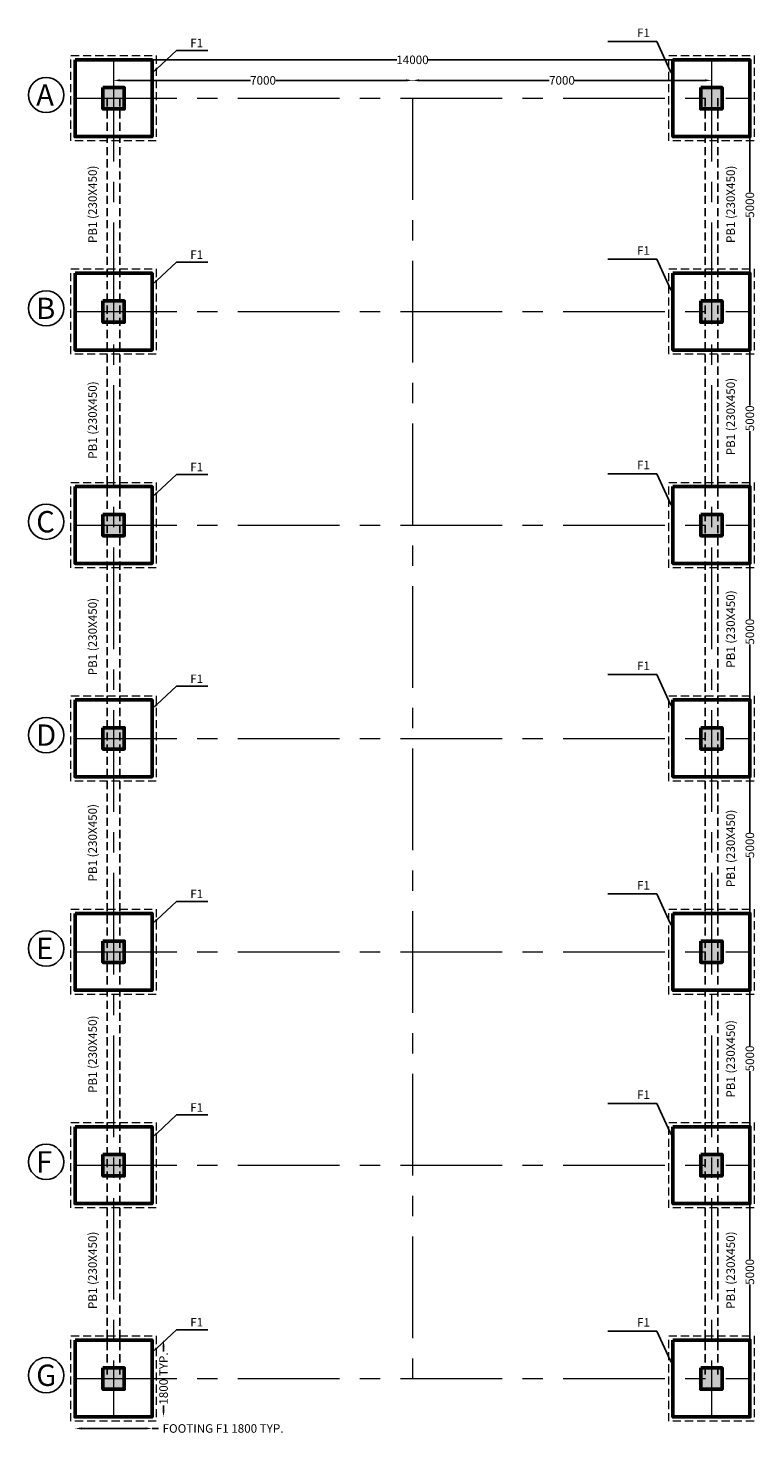
# Model space of a CAD drawing. Units: millimetres. Extents: x -106221 to -52078, y 251365 to 289027.
# Tile 1 of 2: x -106221 to -89199, y 251365 to 284801. Entities that reach past the tile are written whole.
import ezdxf
from ezdxf import colors
from ezdxf.entities.mleader import LeaderData, LeaderLine
from ezdxf.math import Vec2, Vec3

# ---------------------------------------------------------------- set-up
doc = ezdxf.new("R2010")
doc.units = ezdxf.units.MM
doc.header["$LTSCALE"] = 15
doc.header["$MEASUREMENT"] = 0
doc.linetypes.add('CENTER', pattern=[50.8, 31.75, -6.35, 6.35, -6.35])
doc.linetypes.add('DASHED', pattern=[19.05, 12.7, -6.35])
for name, color, linetype, lineweight in [('S-ANNO-DIMS', 2, 'Continuous', 18), ('S-ANNO-TEXT', 7, 'Continuous', 25), ('S-BEAM', 3, 'DASHED', 25), ('S-FNDN', 7, 'Continuous', 50), ('S-FNDN-PCC', 8, 'DASHED', 18), ('S-GRID', 8, 'CENTER', 18), ('S-GRID-IDEN', 7, 'Continuous', 25)]:
    doc.layers.add(name, color=color, linetype=linetype, lineweight=lineweight)
doc.styles.get("Standard").update_dxf_attribs({"font": 'arial.ttf'})
doc.dimstyles.get("Standard").update_dxf_attribs({"dimtxt": 200, "dimasz": 150, "dimexe": 0.18, "dimexo": 0.0625, "dimgap": 0.09, "dimtad": 0, "dimdec": 0, "dimzin": 0, "dimdsep": 46, "dimtxsty": 'Standard', "dimcen": 0.09, "dimadec": 0, "dimazin": 0, "dimtfac": 1, "dimtdec": 0, "dimtofl": 0, "dimtmove": 0, "dimatfit": 3, "dimfxl": 1, "dimfxlon": 1, "dimtolj": 1, "dimtzin": 0, "dimarcsym": 0})

# ---------------------------------------------------------------- blocks, each defined once
blk = doc.blocks.new('*D1')
at = {"layer": 'Defpoints', "color": 0, "ltscale": 15, "transparency": 16777216}
for p in [(-104230, 284068), (-90230, 284068), (-90230, 284068)]:
    blk.add_point(p, dxfattribs=at)
at = {"layer": 'S-ANNO-DIMS', "color": 0, "lineweight": -2, "ltscale": 15, "transparency": 16777216}
for p, q in [((-104230, 284068), (-104230, 284068)), ((-104080, 284068), (-97596, 284068)), ((-90380, 284068), (-96863, 284068)), ((-90230, 284068), (-90230, 284068))]:
    blk.add_line(p, q, dxfattribs=at)
at = {"layer": 'S-ANNO-DIMS', "color": 0, "ltscale": 15, "transparency": 16777216}
for points in [[(-104080, 284093), (-104080, 284043), (-104230, 284068)], [(-90380, 284093), (-90380, 284043), (-90230, 284068)]]:
    blk.add_solid(points, dxfattribs=at)
at = {"layer": 'S-ANNO-DIMS', "color": 0, "ltscale": 15, "transparency": 16777216, "insert": (-97230, 284068), "char_height": 200, "attachment_point": 5}
blk.add_mtext('\\A1;14000', dxfattribs=at)
blk = doc.blocks.new('*D2')
at = {"layer": 'Defpoints', "color": 0, "ltscale": 15, "transparency": 16777216}
for p in [(-104230, 283539), (-97230, 283587), (-97230, 283168)]:
    blk.add_point(p, dxfattribs=at)
at = {"layer": 'S-ANNO-DIMS', "color": 0, "lineweight": -2, "ltscale": 15, "transparency": 16777216}
for p, q in [((-104230, 283586), (-104230, 283587)), ((-104080, 283587), (-101027, 283587)), ((-97380, 283587), (-100432, 283587)), ((-97230, 283586), (-97230, 283587))]:
    blk.add_line(p, q, dxfattribs=at)
at = {"layer": 'S-ANNO-DIMS', "color": 0, "ltscale": 15, "transparency": 16777216}
for points in [[(-104080, 283612), (-104080, 283562), (-104230, 283587)], [(-97380, 283612), (-97380, 283562), (-97230, 283587)]]:
    blk.add_solid(points, dxfattribs=at)
at = {"layer": 'S-ANNO-DIMS', "color": 0, "ltscale": 15, "transparency": 16777216, "insert": (-100730, 283587), "char_height": 200, "attachment_point": 5}
blk.add_mtext('\\A1;7000', dxfattribs=at)
blk = doc.blocks.new('*D3')
at = {"layer": 'Defpoints', "color": 0, "ltscale": 15, "transparency": 16777216}
for p in [(-90230, 283587), (-90230, 283418), (-97230, 283168)]:
    blk.add_point(p, dxfattribs=at)
at = {"layer": 'S-ANNO-DIMS', "color": 0, "lineweight": -2, "ltscale": 15, "transparency": 16777216}
for p, q in [((-97230, 283586), (-97230, 283588)), ((-97080, 283587), (-94027, 283587)), ((-90380, 283587), (-93432, 283587)), ((-90230, 283586), (-90230, 283588))]:
    blk.add_line(p, q, dxfattribs=at)
at = {"layer": 'S-ANNO-DIMS', "color": 0, "ltscale": 15, "transparency": 16777216}
for points in [[(-97080, 283612), (-97080, 283562), (-97230, 283587)], [(-90380, 283612), (-90380, 283562), (-90230, 283587)]]:
    blk.add_solid(points, dxfattribs=at)
at = {"layer": 'S-ANNO-DIMS', "color": 0, "ltscale": 15, "transparency": 16777216, "insert": (-93730, 283587), "char_height": 200, "attachment_point": 5}
blk.add_mtext('\\A1;7000', dxfattribs=at)
blk = doc.blocks.new('*D4')
at = {"layer": 'Defpoints', "color": 0, "ltscale": 15, "transparency": 16777216}
for p in [(-89330, 283168), (-89330, 278168), (-89330, 278168)]:
    blk.add_point(p, dxfattribs=at)
at = {"layer": 'S-ANNO-DIMS', "color": 0, "lineweight": -2, "ltscale": 15, "transparency": 16777216}
for p, q in [((-89330, 283168), (-89330, 283168)), ((-89330, 283018), (-89330, 280966)), ((-89330, 278318), (-89330, 280369)), ((-89330, 278168), (-89330, 278168))]:
    blk.add_line(p, q, dxfattribs=at)
at = {"layer": 'S-ANNO-DIMS', "color": 0, "ltscale": 15, "transparency": 16777216}
for points in [[(-89355, 283018), (-89305, 283018), (-89330, 283168)], [(-89355, 278318), (-89305, 278318), (-89330, 278168)]]:
    blk.add_solid(points, dxfattribs=at)
at = {"layer": 'S-ANNO-DIMS', "color": 0, "ltscale": 15, "transparency": 16777216, "insert": (-89330, 280668), "char_height": 200, "attachment_point": 5, "rotation": 90}
blk.add_mtext('\\A1;5000', dxfattribs=at)
blk = doc.blocks.new('*D5')
at = {"layer": 'Defpoints', "color": 0, "ltscale": 15, "transparency": 16777216}
for p in [(-89330, 278168), (-89330, 273168), (-89330, 273168)]:
    blk.add_point(p, dxfattribs=at)
at = {"layer": 'S-ANNO-DIMS', "color": 0, "lineweight": -2, "ltscale": 15, "transparency": 16777216}
for p, q in [((-89330, 278168), (-89330, 278168)), ((-89330, 278018), (-89330, 275966)), ((-89330, 273318), (-89330, 275369)), ((-89330, 273168), (-89330, 273168))]:
    blk.add_line(p, q, dxfattribs=at)
at = {"layer": 'S-ANNO-DIMS', "color": 0, "ltscale": 15, "transparency": 16777216}
for points in [[(-89355, 278018), (-89305, 278018), (-89330, 278168)], [(-89355, 273318), (-89305, 273318), (-89330, 273168)]]:
    blk.add_solid(points, dxfattribs=at)
at = {"layer": 'S-ANNO-DIMS', "color": 0, "ltscale": 15, "transparency": 16777216, "insert": (-89330, 275668), "char_height": 200, "attachment_point": 5, "rotation": 90}
blk.add_mtext('\\A1;5000', dxfattribs=at)
blk = doc.blocks.new('*D6')
at = {"layer": 'Defpoints', "color": 0, "ltscale": 15, "transparency": 16777216}
for p in [(-89330, 273168), (-89330, 268168), (-89330, 268168)]:
    blk.add_point(p, dxfattribs=at)
at = {"layer": 'S-ANNO-DIMS', "color": 0, "lineweight": -2, "ltscale": 15, "transparency": 16777216}
for p, q in [((-89330, 273168), (-89330, 273168)), ((-89330, 273018), (-89330, 270966)), ((-89330, 268318), (-89330, 270369)), ((-89330, 268168), (-89330, 268168))]:
    blk.add_line(p, q, dxfattribs=at)
at = {"layer": 'S-ANNO-DIMS', "color": 0, "ltscale": 15, "transparency": 16777216}
for points in [[(-89355, 273018), (-89305, 273018), (-89330, 273168)], [(-89355, 268318), (-89305, 268318), (-89330, 268168)]]:
    blk.add_solid(points, dxfattribs=at)
at = {"layer": 'S-ANNO-DIMS', "color": 0, "ltscale": 15, "transparency": 16777216, "insert": (-89330, 270668), "char_height": 200, "attachment_point": 5, "rotation": 90}
blk.add_mtext('\\A1;5000', dxfattribs=at)
blk = doc.blocks.new('*D7')
at = {"layer": 'Defpoints', "color": 0, "ltscale": 15, "transparency": 16777216}
for p in [(-89330, 268168), (-89330, 263168), (-89330, 263168)]:
    blk.add_point(p, dxfattribs=at)
at = {"layer": 'S-ANNO-DIMS', "color": 0, "lineweight": -2, "ltscale": 15, "transparency": 16777216}
for p, q in [((-89330, 268168), (-89330, 268168)), ((-89330, 268018), (-89330, 265966)), ((-89330, 263318), (-89330, 265369)), ((-89330, 263168), (-89330, 263168))]:
    blk.add_line(p, q, dxfattribs=at)
at = {"layer": 'S-ANNO-DIMS', "color": 0, "ltscale": 15, "transparency": 16777216}
for points in [[(-89355, 268018), (-89305, 268018), (-89330, 268168)], [(-89355, 263318), (-89305, 263318), (-89330, 263168)]]:
    blk.add_solid(points, dxfattribs=at)
at = {"layer": 'S-ANNO-DIMS', "color": 0, "ltscale": 15, "transparency": 16777216, "insert": (-89330, 265668), "char_height": 200, "attachment_point": 5, "rotation": 90}
blk.add_mtext('\\A1;5000', dxfattribs=at)
blk = doc.blocks.new('*D8')
at = {"layer": 'Defpoints', "color": 0, "ltscale": 15, "transparency": 16777216}
for p in [(-89330, 263168), (-89330, 258168), (-89330, 258168)]:
    blk.add_point(p, dxfattribs=at)
at = {"layer": 'S-ANNO-DIMS', "color": 0, "lineweight": -2, "ltscale": 15, "transparency": 16777216}
for p, q in [((-89330, 263168), (-89330, 263168)), ((-89330, 263018), (-89330, 260966)), ((-89330, 258318), (-89330, 260369)), ((-89330, 258168), (-89330, 258168))]:
    blk.add_line(p, q, dxfattribs=at)
at = {"layer": 'S-ANNO-DIMS', "color": 0, "ltscale": 15, "transparency": 16777216}
for points in [[(-89355, 263018), (-89305, 263018), (-89330, 263168)], [(-89355, 258318), (-89305, 258318), (-89330, 258168)]]:
    blk.add_solid(points, dxfattribs=at)
at = {"layer": 'S-ANNO-DIMS', "color": 0, "ltscale": 15, "transparency": 16777216, "insert": (-89330, 260668), "char_height": 200, "attachment_point": 5, "rotation": 90}
blk.add_mtext('\\A1;5000', dxfattribs=at)
blk = doc.blocks.new('*D9')
at = {"layer": 'Defpoints', "color": 0, "ltscale": 15, "transparency": 16777216}
for p in [(-89330, 258168), (-89330, 253168), (-89330, 253168)]:
    blk.add_point(p, dxfattribs=at)
at = {"layer": 'S-ANNO-DIMS', "color": 0, "lineweight": -2, "ltscale": 15, "transparency": 16777216}
for p, q in [((-89330, 258168), (-89330, 258168)), ((-89330, 258018), (-89330, 255966)), ((-89330, 253318), (-89330, 255369)), ((-89330, 253168), (-89330, 253168))]:
    blk.add_line(p, q, dxfattribs=at)
at = {"layer": 'S-ANNO-DIMS', "color": 0, "ltscale": 15, "transparency": 16777216}
for points in [[(-89355, 258018), (-89305, 258018), (-89330, 258168)], [(-89355, 253318), (-89305, 253318), (-89330, 253168)]]:
    blk.add_solid(points, dxfattribs=at)
at = {"layer": 'S-ANNO-DIMS', "color": 0, "ltscale": 15, "transparency": 16777216, "insert": (-89330, 255668), "char_height": 200, "attachment_point": 5, "rotation": 90}
blk.add_mtext('\\A1;5000', dxfattribs=at)
blk = doc.blocks.new('FOOTING-F1')
h = blk.add_hatch(color=256)
h.dxf.hatch_style = 1
h.paths.add_polyline_path([(1150, 1150), (650, 1150), (650, 650), (1150, 650)])
for points in [[(0, 1800), (1800, 1800), (1800, 0), (0, 0)], [(650, 1150), (1150, 1150), (1150, 650), (650, 650)]]:
    blk.add_lwpolyline(points, close=True)
blk = doc.blocks.new('*D13')
at = {"layer": 'Defpoints', "color": 0, "ltscale": 15, "transparency": 16777216}
for p in [(-105130, 252268), (-103330, 252268), (-103330, 251998)]:
    blk.add_point(p, dxfattribs=at)
at = {"layer": 'S-ANNO-DIMS', "color": 0, "lineweight": -2, "ltscale": 15, "transparency": 16777216}
for p, q in [((-105130, 251999), (-105130, 251997)), ((-104980, 251998), (-103480, 251998)), ((-103330, 251999), (-103330, 251997)), ((-103330, 251998), (-103180, 251998))]:
    blk.add_line(p, q, dxfattribs=at)
at = {"layer": 'S-ANNO-DIMS', "color": 0, "ltscale": 15, "transparency": 16777216}
for points in [[(-104980, 252023), (-104980, 251973), (-105130, 251998)], [(-103480, 252023), (-103480, 251973), (-103330, 251998)]]:
    blk.add_solid(points, dxfattribs=at)
at = {"layer": 'S-ANNO-DIMS', "color": 0, "ltscale": 15, "transparency": 16777216, "insert": (-101666, 251998), "char_height": 200, "attachment_point": 5}
blk.add_mtext('\\A1;FOOTING F1 1800 TYP.', dxfattribs=at)
blk = doc.blocks.new('*D14')
at = {"layer": 'Defpoints', "color": 0, "ltscale": 15, "transparency": 16777216}
for p in [(-103330, 254068), (-103060, 254068), (-103330, 252268)]:
    blk.add_point(p, dxfattribs=at)
at = {"layer": 'S-ANNO-DIMS', "color": 0, "lineweight": -2, "ltscale": 15, "transparency": 16777216}
for p, q in [((-103061, 254068), (-103060, 254068)), ((-103060, 253918), (-103060, 253800)), ((-103060, 252418), (-103060, 252535)), ((-103061, 252268), (-103060, 252268))]:
    blk.add_line(p, q, dxfattribs=at)
at = {"layer": 'S-ANNO-DIMS', "color": 0, "ltscale": 15, "transparency": 16777216}
for points in [[(-103085, 253918), (-103035, 253918), (-103060, 254068)], [(-103085, 252418), (-103035, 252418), (-103060, 252268)]]:
    blk.add_solid(points, dxfattribs=at)
at = {"layer": 'S-ANNO-DIMS', "color": 0, "ltscale": 15, "transparency": 16777216, "insert": (-103060, 253168), "char_height": 200, "attachment_point": 5, "rotation": 90}
blk.add_mtext('\\A1;1800 TYP.', dxfattribs=at)

msp = doc.modelspace()

# ---------------------------------------------------------------- linework, layer by layer
at = {"layer": 'S-BEAM'}
for p, q in [((-104379.8, 283167.6), (-104379.8, 253167.6)), ((-104079.8, 283167.6), (-104079.8, 253167.6)), ((-90379.8, 283167.6), (-90379.8, 253167.6)), ((-90079.8, 283167.6), (-90079.8, 253167.6))]:
    msp.add_line(p, q, dxfattribs=at)
at = {"layer": 'S-FNDN-PCC'}
for points in [[(-105229.8, 284167.6), (-103229.8, 284167.6), (-103229.8, 282167.6), (-105229.8, 282167.6)], [(-91229.8, 284167.6), (-89229.8, 284167.6), (-89229.8, 282167.6), (-91229.8, 282167.6)], [(-105229.8, 279167.6), (-103229.8, 279167.6), (-103229.8, 277167.6), (-105229.8, 277167.6)], [(-91229.8, 279167.6), (-89229.8, 279167.6), (-89229.8, 277167.6), (-91229.8, 277167.6)], [(-105229.8, 274167.6), (-103229.8, 274167.6), (-103229.8, 272167.6), (-105229.8, 272167.6)], [(-91229.8, 274167.6), (-89229.8, 274167.6), (-89229.8, 272167.6), (-91229.8, 272167.6)], [(-105229.8, 269167.6), (-103229.8, 269167.6), (-103229.8, 267167.6), (-105229.8, 267167.6)], [(-91229.8, 269167.6), (-89229.8, 269167.6), (-89229.8, 267167.6), (-91229.8, 267167.6)], [(-105229.8, 264167.6), (-103229.8, 264167.6), (-103229.8, 262167.6), (-105229.8, 262167.6)], [(-91229.8, 264167.6), (-89229.8, 264167.6), (-89229.8, 262167.6), (-91229.8, 262167.6)], [(-105229.8, 259167.6), (-103229.8, 259167.6), (-103229.8, 257167.6), (-105229.8, 257167.6)], [(-91229.8, 259167.6), (-89229.8, 259167.6), (-89229.8, 257167.6), (-91229.8, 257167.6)], [(-105229.8, 254167.6), (-103229.8, 254167.6), (-103229.8, 252167.6), (-105229.8, 252167.6)], [(-91229.8, 254167.6), (-89229.8, 254167.6), (-89229.8, 252167.6), (-91229.8, 252167.6)]]:
    msp.add_lwpolyline(points, close=True, dxfattribs=at)
at = {"layer": 'S-GRID', "ltscale": 5}
for p, q in [((-104229.8, 284067.6), (-104229.8, 252267.6)), ((-90229.8, 284067.6), (-90229.8, 252267.6)), ((-105129.8, 283167.6), (-89329.8, 283167.6)), ((-97229.8, 283167.6), (-97229.8, 253167.6)), ((-105129.8, 278167.6), (-89329.8, 278167.6)), ((-105129.8, 273167.6), (-89329.8, 273167.6)), ((-105129.8, 268167.6), (-89329.8, 268167.6)), ((-105129.8, 263167.6), (-89329.8, 263167.6)), ((-105129.8, 258167.6), (-89329.8, 258167.6)), ((-105129.8, 253167.6), (-89329.8, 253167.6))]:
    msp.add_line(p, q, dxfattribs=at)
at = {"layer": 'S-GRID-IDEN', "ltscale": 15}
for centre in [(-105808.1, 283244.8), (-105808.1, 278244.8), (-105808.1, 273244.8), (-105808.1, 268244.8), (-105808.1, 263244.8), (-105808.1, 258244.8), (-105808.1, 253244.8)]:
    msp.add_circle(centre, 412.7, dxfattribs=at)

# ---------------------------------------------------------------- block references
at = {"layer": 'S-FNDN'}
for p in [(-105129.8, 282267.6), (-91129.8, 282267.6), (-105129.8, 277267.6), (-91129.8, 277267.6), (-105129.8, 272267.6), (-91129.8, 272267.6), (-105129.8, 267267.6), (-91129.8, 267267.6), (-105129.8, 262267.6), (-91129.8, 262267.6), (-105129.8, 257267.6), (-91129.8, 257267.6), (-105129.8, 252267.6), (-91129.8, 252267.6)]:
    msp.add_blockref('FOOTING-F1', p, dxfattribs=at)

# ---------------------------------------------------------------- texts
at = {"layer": 'S-ANNO-TEXT', "ltscale": 15, "char_height": 200, "attachment_point": 1}
for insert in [(-102433.5, 284563.6), (-91971.3, 284801.1), (-102433.5, 279602.9), (-91971.3, 279699.1), (-102433.5, 274625.6), (-91971.3, 274673.2), (-91971.3, 269967.3), (-102433.5, 269664.7), (-91971.3, 264826.8), (-102433.5, 264624.6), (-91971.3, 259917.2), (-102433.5, 259619.1), (-102433.5, 254587.4), (-91971.3, 254582.9)]:
    msp.add_mtext_dynamic_manual_height_columns('F1', width=2119.366, gutter_width=1, heights=[262.2], dxfattribs=dict(at, insert=insert))
at = {"layer": 'S-ANNO-TEXT', "ltscale": 15, "char_height": 200, "attachment_point": 1, "rotation": 90}
for insert in [(-104821.9, 279775.3), (-89879.1, 279775.3), (-89879.1, 274801.3), (-104821.9, 274720.4), (-89879.1, 269822.9), (-104821.9, 269645.2), (-104821.9, 264816), (-89879.1, 264683.7), (-104821.9, 259859.8), (-89879.1, 259750.9), (-104821.9, 254796), (-89879.1, 254800.4)]:
    msp.add_mtext_dynamic_manual_height_columns('PB1 (230X450)', width=2119.366, gutter_width=1, heights=[0], dxfattribs=dict(at, insert=insert))
at = {"layer": 'S-GRID-IDEN', "ltscale": 15, "char_height": 500, "attachment_point": 1}
for s, insert in [('A', (-106041.6, 283494.8)), ('B', (-106041.6, 278494.8)), ('C', (-106041.6, 273494.8)), ('D', (-106041.6, 268494.8)), ('E', (-106041.6, 263494.8)), ('F', (-106041.6, 258494.8)), ('G', (-106041.6, 253494.8))]:
    msp.add_mtext_dynamic_manual_height_columns(s, width=500, gutter_width=1, heights=[0], dxfattribs=dict(at, insert=insert))

# ---------------------------------------------------------------- dimensions: what is measured, and where the dimension line sits
at = {"layer": 'S-ANNO-DIMS', "ltscale": 15}
for base, p1, p2, picture, middle in [((-90229.8, 284067.6), (-104229.8, 284067.6), (-90229.8, 284067.6), '*D1', (-97229.8, 284067.6)), ((-97229.8, 283587.3), (-104229.8, 283538.9), (-97229.8, 283167.6), '*D2', (-100729.8, 283587.3)), ((-90229.8, 283587.4), (-97229.8, 283167.6), (-90229.8, 283417.6), '*D3', (-93729.8, 283587.4))]:
    dim = msp.add_linear_dim(base=base, p1=p1, p2=p2, dimstyle='Standard', override={"dimclrd": 0, "dimclre": 0, "dimclrt": 0}, dxfattribs=at)
    dim.commit()
    dim.dimension.update_dxf_attribs({"geometry": picture, "text_midpoint": middle})
for base, p1, p2, picture, middle in [((-89329.8, 278167.6), (-89329.8, 283167.6), (-89329.8, 278167.6), '*D4', (-89329.8, 280667.6)), ((-89329.8, 273167.6), (-89329.8, 278167.6), (-89329.8, 273167.6), '*D5', (-89329.8, 275667.6)), ((-89329.8, 268167.6), (-89330, 273167.6), (-89329.8, 268167.6), '*D6', (-89329.8, 270667.6)), ((-89329.8, 263167.6), (-89330, 268167.6), (-89329.8, 263167.6), '*D7', (-89329.8, 265667.6)), ((-89329.8, 258167.6), (-89330, 263167.6), (-89329.8, 258167.6), '*D8', (-89329.8, 260667.6)), ((-89329.8, 253167.6), (-89329.8, 258167.6), (-89329.8, 253167.6), '*D9', (-89329.8, 255667.6))]:
    dim = msp.add_linear_dim(base=base, p1=p1, p2=p2, angle=90, dimstyle='Standard', override={"dimclrd": 0, "dimclre": 0, "dimclrt": 0}, dxfattribs=at)
    dim.commit()
    dim.dimension.update_dxf_attribs({"geometry": picture, "text_midpoint": middle})
dim = msp.add_linear_dim(base=(-103059.8, 254067.6), p1=(-103329.8, 252267.6), p2=(-103329.8, 254067.6), angle=90, text='<> TYP.', dimstyle='Standard', override={"dimdec": 0, "dimlfac": 1, "dimrnd": 0, "dimzin": 0, "dimdsep": 46, "dimlunit": 2}, dxfattribs=at)
dim.commit()
dim.dimension.update_dxf_attribs({"geometry": '*D14', "text_midpoint": (-103059.8, 253167.6)})
dim = msp.add_linear_dim(base=(-103329.8, 251997.6), p1=(-105129.8, 252267.6), p2=(-103329.8, 252267.6), text='FOOTING F1 <> TYP.', dimstyle='Standard', override={"dimdec": 0, "dimlfac": 1, "dimrnd": 0, "dimzin": 0, "dimdsep": 46, "dimlunit": 2}, dxfattribs=at)
dim.commit()
dim.dimension.update_dxf_attribs({"geometry": '*D13', "text_midpoint": (-101666.2, 251997.6)})

# ---------------------------------------------------------------- leaders
at = {"layer": 'S-ANNO-TEXT', "ltscale": 15}
ml = msp.add_multileader_mtext('Standard', dxfattribs=at)
ml.set_content('', color=256)
ml.set_leader_properties()
ml.build(insert=Vec2(0, 0))
ml.multileader.update_dxf_attribs({"dogleg_length": 0.36, "arrow_head_size": 150})
ctx = ml.context
ctx.base_point, ctx.char_height, ctx.arrow_head_size, ctx.landing_gap_size, ctx.plane_origin = Vec3(-92653.8, 284496.7), 200, 150, 0.09, Vec3(-91129.8, 283677.2)
ctx.text_align_type = 2
notes = []
notes.append((ctx, [(0, (1, 1, 0), (-92653.3, 284496.7), (-1, 0), 0.36, [(0, [(-91129.8, 283677.2), (-91506.8, 284496.7)], 0, [])])]))
ctx.mtext.insert, ctx.mtext.alignment, ctx.mtext.flow_direction = Vec3(-92653.7, 284596.7), 3, 5
ml = msp.add_multileader_mtext('Standard', dxfattribs=at)
ml.set_content('', color=256)
ml.set_leader_properties()
ml.build(insert=Vec2(0, 0))
ml.multileader.update_dxf_attribs({"dogleg_length": 0.36, "arrow_head_size": 150})
ctx = ml.context
ctx.base_point, ctx.char_height, ctx.arrow_head_size, ctx.landing_gap_size, ctx.plane_origin = Vec3(-102021.6, 284288.2), 200, 150, 0.09, Vec3(-103329.8, 283755.4)
notes.append((ctx, [(0, (1, 1, 0), (-102021.9, 284288.2), (1, 0), 0.36, [(0, [(-103329.8, 283755.4), (-102758.2, 284288.2)], 0, [])])]))
ctx.mtext.insert, ctx.mtext.flow_direction = Vec3(-102021.5, 284388.2), 5
ml = msp.add_multileader_mtext('Standard', dxfattribs=at)
ml.set_content('', color=256)
ml.set_leader_properties()
ml.build(insert=Vec2(0, 0))
ml.multileader.update_dxf_attribs({"dogleg_length": 0.36, "arrow_head_size": 150})
ctx = ml.context
ctx.base_point, ctx.char_height, ctx.arrow_head_size, ctx.landing_gap_size, ctx.plane_origin = Vec3(-102021.6, 279327.6), 200, 150, 0.09, Vec3(-103329.8, 278794.8)
notes.append((ctx, [(0, (1, 1, 0), (-102021.9, 279327.6), (1, 0), 0.36, [(0, [(-103329.8, 278794.8), (-102758.2, 279327.6)], 0, [])])]))
ctx.mtext.insert, ctx.mtext.flow_direction = Vec3(-102021.5, 279427.6), 5
ml = msp.add_multileader_mtext('Standard', dxfattribs=at)
ml.set_content('', color=256)
ml.set_leader_properties()
ml.build(insert=Vec2(0, 0))
ml.multileader.update_dxf_attribs({"dogleg_length": 0.36, "arrow_head_size": 150})
ctx = ml.context
ctx.base_point, ctx.char_height, ctx.arrow_head_size, ctx.landing_gap_size, ctx.plane_origin = Vec3(-92653.8, 279394.7), 200, 150, 0.09, Vec3(-91129.8, 278575.2)
ctx.text_align_type = 2
notes.append((ctx, [(0, (1, 1, 0), (-92653.3, 279394.7), (-1, 0), 0.36, [(0, [(-91129.8, 278575.2), (-91506.8, 279394.7)], 0, [])])]))
ctx.mtext.insert, ctx.mtext.alignment, ctx.mtext.flow_direction = Vec3(-92653.7, 279494.7), 3, 5
ml = msp.add_multileader_mtext('Standard', dxfattribs=at)
ml.set_content('', color=256)
ml.set_leader_properties()
ml.build(insert=Vec2(0, 0))
ml.multileader.update_dxf_attribs({"dogleg_length": 0.36, "arrow_head_size": 150})
ctx = ml.context
ctx.base_point, ctx.char_height, ctx.arrow_head_size, ctx.landing_gap_size, ctx.plane_origin = Vec3(-102021.6, 274350.2), 200, 150, 0.09, Vec3(-103329.8, 273817.4)
notes.append((ctx, [(0, (1, 1, 0), (-102021.9, 274350.2), (1, 0), 0.36, [(0, [(-103329.8, 273817.4), (-102758.2, 274350.2)], 0, [])])]))
ctx.mtext.insert, ctx.mtext.flow_direction = Vec3(-102021.5, 274450.2), 5
ml = msp.add_multileader_mtext('Standard', dxfattribs=at)
ml.set_content('', color=256)
ml.set_leader_properties()
ml.build(insert=Vec2(0, 0))
ml.multileader.update_dxf_attribs({"dogleg_length": 0.36, "arrow_head_size": 150})
ctx = ml.context
ctx.base_point, ctx.char_height, ctx.arrow_head_size, ctx.landing_gap_size, ctx.plane_origin = Vec3(-92653.8, 274368.7), 200, 150, 0.09, Vec3(-91129.8, 273549.3)
ctx.text_align_type = 2
notes.append((ctx, [(0, (1, 1, 0), (-92653.3, 274368.7), (-1, 0), 0.36, [(0, [(-91129.8, 273549.3), (-91506.8, 274368.7)], 0, [])])]))
ctx.mtext.insert, ctx.mtext.alignment, ctx.mtext.flow_direction = Vec3(-92653.7, 274468.7), 3, 5
ml = msp.add_multileader_mtext('Standard', dxfattribs=at)
ml.set_content('', color=256)
ml.set_leader_properties()
ml.build(insert=Vec2(0, 0))
ml.multileader.update_dxf_attribs({"dogleg_length": 0.36, "arrow_head_size": 150})
ctx = ml.context
ctx.base_point, ctx.char_height, ctx.arrow_head_size, ctx.landing_gap_size, ctx.plane_origin = Vec3(-92653.8, 269662.8), 200, 150, 0.09, Vec3(-91129.8, 268843.4)
ctx.text_align_type = 2
notes.append((ctx, [(0, (1, 1, 0), (-92653.3, 269662.8), (-1, 0), 0.36, [(0, [(-91129.8, 268843.4), (-91506.8, 269662.8)], 0, [])])]))
ctx.mtext.insert, ctx.mtext.alignment, ctx.mtext.flow_direction = Vec3(-92653.7, 269762.8), 3, 5
ml = msp.add_multileader_mtext('Standard', dxfattribs=at)
ml.set_content('', color=256)
ml.set_leader_properties()
ml.build(insert=Vec2(0, 0))
ml.multileader.update_dxf_attribs({"dogleg_length": 0.36, "arrow_head_size": 150})
ctx = ml.context
ctx.base_point, ctx.char_height, ctx.arrow_head_size, ctx.landing_gap_size, ctx.plane_origin = Vec3(-102021.6, 269389.4), 200, 150, 0.09, Vec3(-103329.8, 268856.6)
notes.append((ctx, [(0, (1, 1, 0), (-102021.9, 269389.4), (1, 0), 0.36, [(0, [(-103329.8, 268856.6), (-102758.2, 269389.4)], 0, [])])]))
ctx.mtext.insert, ctx.mtext.flow_direction = Vec3(-102021.5, 269489.4), 5
ml = msp.add_multileader_mtext('Standard', dxfattribs=at)
ml.set_content('', color=256)
ml.set_leader_properties()
ml.build(insert=Vec2(0, 0))
ml.multileader.update_dxf_attribs({"dogleg_length": 0.36, "arrow_head_size": 150})
ctx = ml.context
ctx.base_point, ctx.char_height, ctx.arrow_head_size, ctx.landing_gap_size, ctx.plane_origin = Vec3(-92653.8, 264522.3), 200, 150, 0.09, Vec3(-91129.8, 263702.9)
ctx.text_align_type = 2
notes.append((ctx, [(0, (1, 1, 0), (-92653.3, 264522.3), (-1, 0), 0.36, [(0, [(-91129.8, 263702.9), (-91506.8, 264522.3)], 0, [])])]))
ctx.mtext.insert, ctx.mtext.alignment, ctx.mtext.flow_direction = Vec3(-92653.7, 264622.3), 3, 5
ml = msp.add_multileader_mtext('Standard', dxfattribs=at)
ml.set_content('', color=256)
ml.set_leader_properties()
ml.build(insert=Vec2(0, 0))
ml.multileader.update_dxf_attribs({"dogleg_length": 0.36, "arrow_head_size": 150})
ctx = ml.context
ctx.base_point, ctx.char_height, ctx.arrow_head_size, ctx.landing_gap_size, ctx.plane_origin = Vec3(-102021.6, 264349.2), 200, 150, 0.09, Vec3(-103329.8, 263816.4)
notes.append((ctx, [(0, (1, 1, 0), (-102021.9, 264349.2), (1, 0), 0.36, [(0, [(-103329.8, 263816.4), (-102758.2, 264349.2)], 0, [])])]))
ctx.mtext.insert, ctx.mtext.flow_direction = Vec3(-102021.5, 264449.2), 5
ml = msp.add_multileader_mtext('Standard', dxfattribs=at)
ml.set_content('', color=256)
ml.set_leader_properties()
ml.build(insert=Vec2(0, 0))
ml.multileader.update_dxf_attribs({"dogleg_length": 0.36, "arrow_head_size": 150})
ctx = ml.context
ctx.base_point, ctx.char_height, ctx.arrow_head_size, ctx.landing_gap_size, ctx.plane_origin = Vec3(-92653.8, 259612.7), 200, 150, 0.09, Vec3(-91129.8, 258793.3)
ctx.text_align_type = 2
notes.append((ctx, [(0, (1, 1, 0), (-92653.3, 259612.7), (-1, 0), 0.36, [(0, [(-91129.8, 258793.3), (-91506.8, 259612.7)], 0, [])])]))
ctx.mtext.insert, ctx.mtext.alignment, ctx.mtext.flow_direction = Vec3(-92653.7, 259712.7), 3, 5
ml = msp.add_multileader_mtext('Standard', dxfattribs=at)
ml.set_content('', color=256)
ml.set_leader_properties()
ml.build(insert=Vec2(0, 0))
ml.multileader.update_dxf_attribs({"dogleg_length": 0.36, "arrow_head_size": 150})
ctx = ml.context
ctx.base_point, ctx.char_height, ctx.arrow_head_size, ctx.landing_gap_size, ctx.plane_origin = Vec3(-102021.6, 259343.8), 200, 150, 0.09, Vec3(-103329.8, 258811)
notes.append((ctx, [(0, (1, 1, 0), (-102021.9, 259343.8), (1, 0), 0.36, [(0, [(-103329.8, 258811), (-102758.2, 259343.8)], 0, [])])]))
ctx.mtext.insert, ctx.mtext.flow_direction = Vec3(-102021.5, 259443.8), 5
ml = msp.add_multileader_mtext('Standard', dxfattribs=at)
ml.set_content('', color=256)
ml.set_leader_properties()
ml.build(insert=Vec2(0, 0))
ml.multileader.update_dxf_attribs({"dogleg_length": 0.36, "arrow_head_size": 150})
ctx = ml.context
ctx.base_point, ctx.char_height, ctx.arrow_head_size, ctx.landing_gap_size, ctx.plane_origin = Vec3(-102021.6, 254312), 200, 150, 0.09, Vec3(-103329.8, 253779.2)
notes.append((ctx, [(0, (1, 1, 0), (-102021.9, 254312), (1, 0), 0.36, [(0, [(-103329.8, 253779.2), (-102758.2, 254312)], 0, [])])]))
ctx.mtext.insert, ctx.mtext.flow_direction = Vec3(-102021.5, 254412), 5
ml = msp.add_multileader_mtext('Standard', dxfattribs=at)
ml.set_content('', color=256)
ml.set_leader_properties()
ml.build(insert=Vec2(0, 0))
ml.multileader.update_dxf_attribs({"dogleg_length": 0.36, "arrow_head_size": 150})
ctx = ml.context
ctx.base_point, ctx.char_height, ctx.arrow_head_size, ctx.landing_gap_size, ctx.plane_origin = Vec3(-92653.8, 254278.5), 200, 150, 0.09, Vec3(-91129.8, 253459.1)
ctx.text_align_type = 2
notes.append((ctx, [(0, (1, 1, 0), (-92653.3, 254278.5), (-1, 0), 0.36, [(0, [(-91129.8, 253459.1), (-91506.8, 254278.5)], 0, [])])]))
ctx.mtext.insert, ctx.mtext.alignment, ctx.mtext.flow_direction = Vec3(-92653.7, 254378.5), 3, 5
for ctx, leaders in notes:
    for number, flags, end, landing, length, lines in leaders:
        leader = LeaderData()
        leader.index, (leader.has_last_leader_line, leader.has_dogleg_vector, leader.attachment_direction) = number, flags
        leader.last_leader_point, leader.dogleg_vector, leader.dogleg_length = Vec3(end), Vec3(landing), length
        for number, points, colour, breaks in lines:
            line = LeaderLine()
            line.index, line.vertices, line.color, line.breaks = number, Vec3.list(points), colors.encode_raw_color(colour), breaks
            leader.lines.append(line)
        ctx.leaders.append(leader)

doc.saveas('drawing.dxf')
